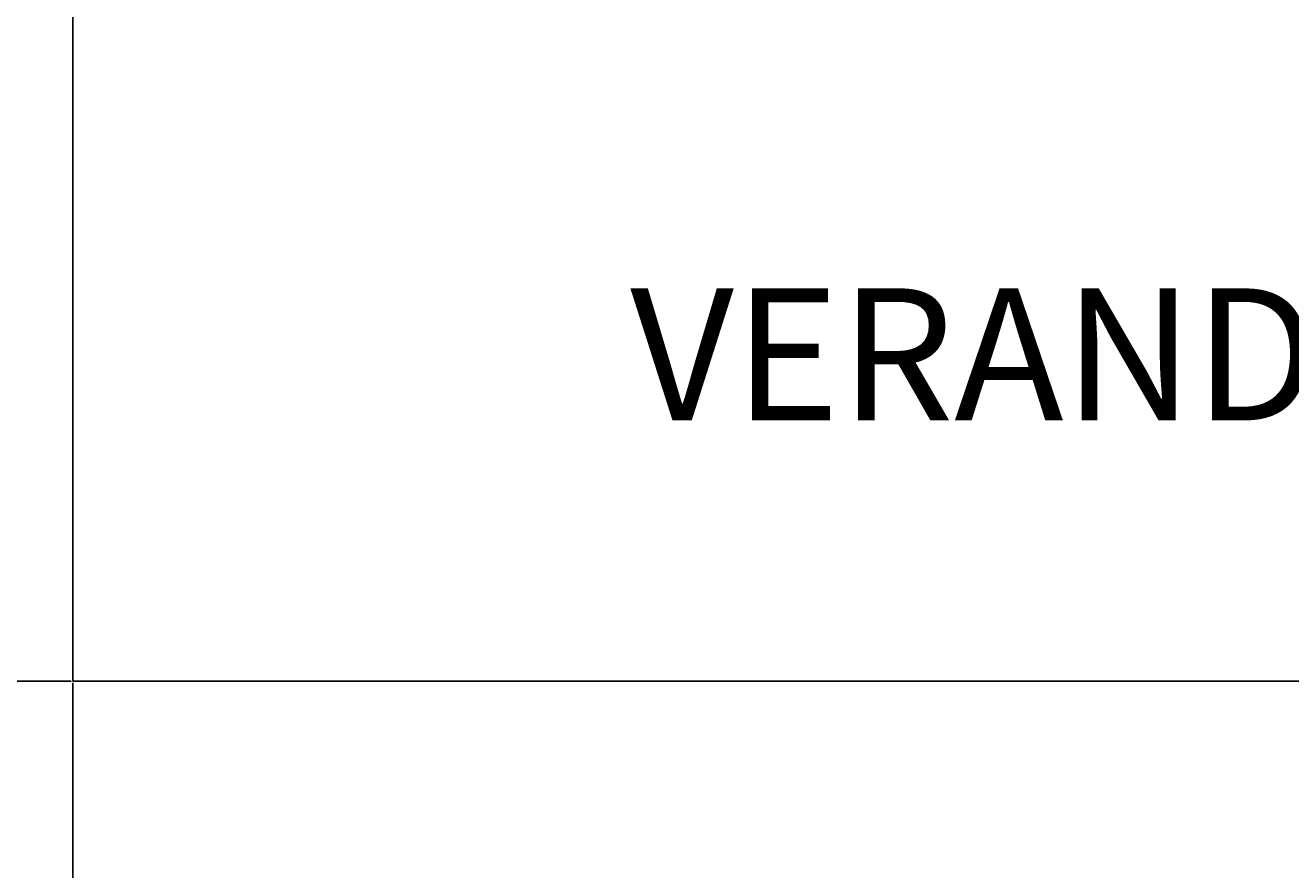
# Model space of a CAD drawing. Units: inches. Extents: x 1885 to 2748, y 783 to 2421.
# Tile 3 of 117: x 1969 to 2017, y 1050 to 1082. Entities that reach past the tile are written whole.
import ezdxf

# ---------------------------------------------------------------- set-up
doc = ezdxf.new("R2010")
doc.units = ezdxf.units.IN
for name, color, linetype, lineweight in [('A-ANNO-DIMS', 2, 'Continuous', 18), ('A-AREA-IDEN', 7, 'Continuous', 18), ('A-FLOR-BALC', 7, 'Continuous', 25)]:
    doc.layers.add(name, color=color, linetype=linetype, lineweight=lineweight)
doc.styles.get("Standard").update_dxf_attribs({"font": 'arial.ttf'})
doc.dimstyles.get("Standard").update_dxf_attribs({"dimtxt": 0.18, "dimasz": 0.18, "dimexe": 0.18, "dimexo": 0.0625, "dimgap": 0.09, "dimtad": 0, "dimtih": 1, "dimtoh": 1, "dimdec": 4, "dimzin": 0, "dimdsep": 46, "dimtxsty": 'Standard', "dimcen": 0.09, "dimadec": 0, "dimazin": 0, "dimtfac": 1, "dimtdec": 4, "dimtofl": 0, "dimtmove": 0, "dimatfit": 3, "dimfxl": 1, "dimtolj": 1, "dimtzin": 0, "dimarcsym": 0})

# ---------------------------------------------------------------- blocks, each defined once
blk = doc.blocks.new('*D43')
at = {"layer": 'A-ANNO-DIMS', "color": 0, "lineweight": -2, "transparency": 16777216}
for p, q in [((1971.274, 1057.443), (1971.274, 922.479)), ((2618.274, 1057.443), (2618.274, 922.479)), ((1971.454, 922.659), (2294.484, 922.659)), ((2618.094, 922.659), (2295.063, 922.659))]:
    blk.add_line(p, q, dxfattribs=at)
at = {"layer": 'A-ANNO-DIMS', "color": 0, "transparency": 16777216}
for points in [[(1971.454, 922.689), (1971.454, 922.629), (1971.274, 922.659)], [(2618.094, 922.689), (2618.094, 922.629), (2618.274, 922.659)]]:
    blk.add_solid(points, dxfattribs=at)
at = {"layer": 'Defpoints', "color": 0, "transparency": 16777216}
for p in [(1971.274, 1057.506), (2618.274, 1057.506), (2618.274, 922.659)]:
    blk.add_point(p, dxfattribs=at)
at = {"layer": 'A-ANNO-DIMS', "color": 0, "transparency": 16777216, "insert": (2294.774, 922.659), "char_height": 0.18, "attachment_point": 5}
blk.add_mtext('\\A1;647', dxfattribs=at)
blk = doc.blocks.new('*D45')
at = {"layer": 'A-ANNO-DIMS', "color": 0, "lineweight": -2, "transparency": 16777216}
for p, q in [((1980.711, 1524.006), (1902.844, 1524.006)), ((1903.024, 1523.826), (1903.024, 1290.937)), ((1903.024, 1057.686), (1903.024, 1290.574)), ((1971.211, 1057.506), (1902.844, 1057.506))]:
    blk.add_line(p, q, dxfattribs=at)
at = {"layer": 'A-ANNO-DIMS', "color": 0, "transparency": 16777216}
for points in [[(1902.994, 1523.826), (1903.054, 1523.826), (1903.024, 1524.006)], [(1902.994, 1057.686), (1903.054, 1057.686), (1903.024, 1057.506)]]:
    blk.add_solid(points, dxfattribs=at)
at = {"layer": 'Defpoints', "color": 0, "transparency": 16777216}
for p in [(1903.024, 1524.006), (1980.774, 1524.006), (1971.274, 1057.506)]:
    blk.add_point(p, dxfattribs=at)
at = {"layer": 'A-ANNO-DIMS', "color": 0, "transparency": 16777216, "insert": (1903.024, 1290.756), "char_height": 0.18, "attachment_point": 5}
blk.add_mtext('\\A1;466.5', dxfattribs=at)

msp = doc.modelspace()

# ---------------------------------------------------------------- linework, layer by layer
at = {"layer": 'A-FLOR-BALC'}
for p, q in [((1971.274, 1087.506), (1971.274, 1057.506)), ((1971.274, 1057.506), (2112.274, 1057.506))]:
    msp.add_line(p, q, dxfattribs=at)

# ---------------------------------------------------------------- texts
at = {"layer": 'A-AREA-IDEN', "insert": (1992.384, 1072.38), "char_height": 5, "attachment_point": 1}
msp.add_mtext_dynamic_manual_height_columns('VERANDAH  12\'0"x2\'6"', width=123.4564, gutter_width=12.5, heights=[0], dxfattribs=at)

# ---------------------------------------------------------------- dimensions: what is measured, and where the dimension line sits
at = {"layer": 'A-ANNO-DIMS'}
dim = msp.add_linear_dim(base=(1903.024, 1524.006), p1=(1971.274, 1057.506), p2=(1980.774, 1524.006), angle=90, dimstyle='Standard', override={"dimdec": 1, "dimlfac": 1, "dimrnd": 0, "dimzin": 0, "dimdsep": 46, "dimlunit": 2}, dxfattribs=at)
dim.commit()
dim.dimension.update_dxf_attribs({"geometry": '*D45', "text_midpoint": (1903.024, 1290.756)})
dim = msp.add_linear_dim(base=(2618.274, 922.659), p1=(1971.274, 1057.506), p2=(2618.274, 1057.506), dimstyle='Standard', override={"dimdec": 0, "dimlfac": 1, "dimrnd": 0, "dimzin": 0, "dimdsep": 46, "dimlunit": 2}, dxfattribs=at)
dim.commit()
dim.dimension.update_dxf_attribs({"geometry": '*D43', "text_midpoint": (2294.774, 922.659)})

doc.saveas('drawing.dxf')
